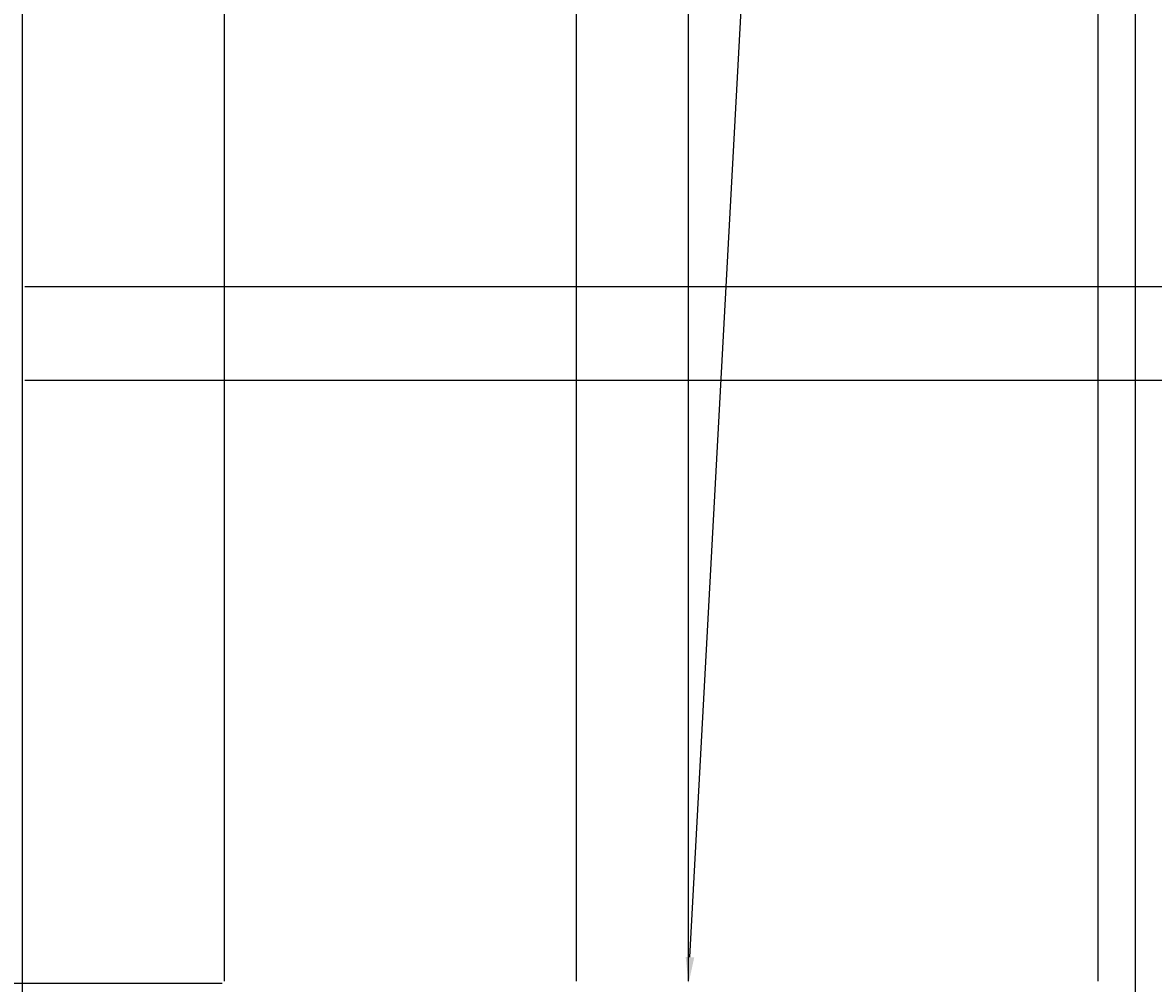
# Model space of a CAD drawing. Units: inches. Extents: x -12 to 334, y -10 to 186.
# Tile 23 of 77: x 58 to 88, y 109 to 135. Entities that reach past the tile are written whole.
import ezdxf
from ezdxf import colors
from ezdxf.entities.mleader import LeaderData, LeaderLine
from ezdxf.math import Vec2, Vec3

# ---------------------------------------------------------------- set-up
doc = ezdxf.new("R2010")
doc.units = ezdxf.units.IN
doc.header["$MEASUREMENT"] = 0
doc.layers.add('M-ANNO-TEXT', color=3, linetype='Continuous', lineweight=25)
doc.layers.add('M-DIMS', color=2, linetype='Continuous', lineweight=18)
doc.styles.get("Standard").update_dxf_attribs({"font": 'arial.ttf'})
doc.dimstyles.get("Standard").update_dxf_attribs({"dimtxt": 0.18, "dimasz": 0.18, "dimexe": 0.18, "dimexo": 0.0625, "dimgap": 0.09, "dimtad": 0, "dimtih": 1, "dimtoh": 1, "dimdec": 4, "dimzin": 0, "dimdsep": 46, "dimtxsty": 'Standard', "dimcen": 0.09, "dimadec": 0, "dimazin": 0, "dimtfac": 1, "dimtdec": 4, "dimtofl": 0, "dimtmove": 0, "dimatfit": 3, "dimfxl": 1, "dimtolj": 1, "dimtzin": 0, "dimarcsym": 0})

# ---------------------------------------------------------------- blocks, each defined once
blk = doc.blocks.new('*D3')
at = {"layer": 'Defpoints', "color": 0, "transparency": 16777216}
for p in [(58.1, 169.385), (32.1, 127.708), (58.1, 127.708)]:
    blk.add_point(p, dxfattribs=at)
at = {"layer": 'M-DIMS', "color": 0, "lineweight": -2, "transparency": 16777216}
for p, q in [((32.1, 127.77), (32.1, 169.565)), ((58.1, 127.77), (58.1, 169.565)), ((32.28, 169.385), (44.88, 169.385)), ((57.92, 169.385), (45.321, 169.385))]:
    blk.add_line(p, q, dxfattribs=at)
at = {"layer": 'M-DIMS', "color": 0, "transparency": 16777216}
for points in [[(32.28, 169.415), (32.28, 169.355), (32.1, 169.385)], [(57.92, 169.415), (57.92, 169.355), (58.1, 169.385)]]:
    blk.add_solid(points, dxfattribs=at)
at = {"layer": 'M-DIMS', "color": 0, "transparency": 16777216, "insert": (45.1, 169.385), "char_height": 0.18, "attachment_point": 5}
blk.add_mtext('\\A1;26', dxfattribs=at)
blk = doc.blocks.new('*D5')
at = {"layer": 'Defpoints', "color": 0, "transparency": 16777216}
for p in [(58.1, 127.708), (58.1, 125.208), (295.976, 125.208)]:
    blk.add_point(p, dxfattribs=at)
at = {"layer": 'M-DIMS', "color": 0, "lineweight": -2, "transparency": 16777216}
for p, q in [((58.163, 127.708), (296.156, 127.708)), ((295.976, 127.528), (295.976, 126.64)), ((295.976, 125.388), (295.976, 126.276)), ((58.163, 125.208), (296.156, 125.208))]:
    blk.add_line(p, q, dxfattribs=at)
at = {"layer": 'M-DIMS', "color": 0, "transparency": 16777216}
for points in [[(295.946, 127.528), (296.006, 127.528), (295.976, 127.708)], [(295.946, 125.388), (296.006, 125.388), (295.976, 125.208)]]:
    blk.add_solid(points, dxfattribs=at)
at = {"layer": 'M-DIMS', "color": 0, "transparency": 16777216, "insert": (295.976, 126.458), "char_height": 0.18, "attachment_point": 5}
blk.add_mtext('\\A1;2.5', dxfattribs=at)
blk = doc.blocks.new('*D10')
at = {"layer": 'Defpoints', "color": 0, "transparency": 16777216}
for p in [(63.5, 169.385), (58.1, 127.708), (63.5, 109.058)]:
    blk.add_point(p, dxfattribs=at)
at = {"layer": 'M-DIMS', "color": 0, "lineweight": -2, "transparency": 16777216}
for p, q in [((58.1, 127.77), (58.1, 169.565)), ((63.5, 109.121), (63.5, 169.565)), ((58.28, 169.385), (60.547, 169.385)), ((63.32, 169.385), (61.054, 169.385))]:
    blk.add_line(p, q, dxfattribs=at)
at = {"layer": 'M-DIMS', "color": 0, "transparency": 16777216}
for points in [[(58.28, 169.415), (58.28, 169.355), (58.1, 169.385)], [(63.32, 169.415), (63.32, 169.355), (63.5, 169.385)]]:
    blk.add_solid(points, dxfattribs=at)
at = {"layer": 'M-DIMS', "color": 0, "transparency": 16777216, "insert": (60.8, 169.385), "char_height": 0.18, "attachment_point": 5}
blk.add_mtext('\\A1;5.4', dxfattribs=at)
blk = doc.blocks.new('*D11')
at = {"layer": 'Defpoints', "color": 0, "transparency": 16777216}
for p in [(72.924, 169.385), (63.5, 109.058), (72.924, 109.058)]:
    blk.add_point(p, dxfattribs=at)
at = {"layer": 'M-DIMS', "color": 0, "lineweight": -2, "transparency": 16777216}
for p, q in [((63.5, 109.121), (63.5, 169.565)), ((72.924, 109.121), (72.924, 169.565)), ((63.68, 169.385), (67.819, 169.385)), ((72.744, 169.385), (68.606, 169.385))]:
    blk.add_line(p, q, dxfattribs=at)
at = {"layer": 'M-DIMS', "color": 0, "transparency": 16777216}
for points in [[(63.68, 169.415), (63.68, 169.355), (63.5, 169.385)], [(72.744, 169.415), (72.744, 169.355), (72.924, 169.385)]]:
    blk.add_solid(points, dxfattribs=at)
at = {"layer": 'M-DIMS', "color": 0, "transparency": 16777216, "insert": (68.212, 169.385), "char_height": 0.18, "attachment_point": 5}
blk.add_mtext('\\A1;9.424', dxfattribs=at)
blk = doc.blocks.new('*D12')
at = {"layer": 'Defpoints', "color": 0, "transparency": 16777216}
for p in [(75.924, 169.385), (72.924, 109.058), (75.924, 109.058)]:
    blk.add_point(p, dxfattribs=at)
at = {"layer": 'M-DIMS', "color": 0, "lineweight": -2, "transparency": 16777216}
for p, q in [((72.924, 109.121), (72.924, 169.565)), ((75.924, 109.121), (75.924, 169.565)), ((73.104, 169.385), (74.275, 169.385)), ((75.744, 169.385), (74.573, 169.385))]:
    blk.add_line(p, q, dxfattribs=at)
at = {"layer": 'M-DIMS', "color": 0, "transparency": 16777216}
for points in [[(73.104, 169.415), (73.104, 169.355), (72.924, 169.385)], [(75.744, 169.415), (75.744, 169.355), (75.924, 169.385)]]:
    blk.add_solid(points, dxfattribs=at)
at = {"layer": 'M-DIMS', "color": 0, "transparency": 16777216, "insert": (74.424, 169.385), "char_height": 0.18, "attachment_point": 5}
blk.add_mtext('\\A1;3', dxfattribs=at)
blk = doc.blocks.new('*D13')
at = {"layer": 'Defpoints', "color": 0, "transparency": 16777216}
for p in [(86.888, 169.385), (75.924, 109.058), (86.888, 109.058)]:
    blk.add_point(p, dxfattribs=at)
at = {"layer": 'M-DIMS', "color": 0, "lineweight": -2, "transparency": 16777216}
for p, q in [((75.924, 109.121), (75.924, 169.565)), ((86.888, 109.121), (86.888, 169.565)), ((76.104, 169.385), (80.951, 169.385)), ((86.708, 169.385), (81.861, 169.385))]:
    blk.add_line(p, q, dxfattribs=at)
at = {"layer": 'M-DIMS', "color": 0, "transparency": 16777216}
for points in [[(76.104, 169.415), (76.104, 169.355), (75.924, 169.385)], [(86.708, 169.415), (86.708, 169.355), (86.888, 169.385)]]:
    blk.add_solid(points, dxfattribs=at)
at = {"layer": 'M-DIMS', "color": 0, "transparency": 16777216, "insert": (81.406, 169.385), "char_height": 0.18, "attachment_point": 5}
blk.add_mtext('\\A1;10.964', dxfattribs=at)
blk = doc.blocks.new('*D14')
at = {"layer": 'Defpoints', "color": 0, "transparency": 16777216}
for p in [(63.5, 109.058), (-11.174, 49.45), (64.207, 49.45)]:
    blk.add_point(p, dxfattribs=at)
at = {"layer": 'M-DIMS', "color": 0, "lineweight": -2, "transparency": 16777216}
for p, q in [((63.438, 109.058), (-11.354, 109.058)), ((-11.174, 108.878), (-11.174, 79.436)), ((-11.174, 49.63), (-11.174, 79.072)), ((64.144, 49.45), (-11.354, 49.45))]:
    blk.add_line(p, q, dxfattribs=at)
at = {"layer": 'M-DIMS', "color": 0, "transparency": 16777216}
for points in [[(-11.204, 108.878), (-11.144, 108.878), (-11.174, 109.058)], [(-11.204, 49.63), (-11.144, 49.63), (-11.174, 49.45)]]:
    blk.add_solid(points, dxfattribs=at)
at = {"layer": 'M-DIMS', "color": 0, "transparency": 16777216, "insert": (-11.174, 79.254), "char_height": 0.18, "attachment_point": 5}
blk.add_mtext('\\A1;59.61', dxfattribs=at)
blk = doc.blocks.new('*D15')
at = {"layer": 'Defpoints', "color": 0, "transparency": 16777216}
for p in [(106.177, 169.385), (86.888, 109.058), (106.177, 102.896)]:
    blk.add_point(p, dxfattribs=at)
at = {"layer": 'M-DIMS', "color": 0, "lineweight": -2, "transparency": 16777216}
for p, q in [((86.888, 109.121), (86.888, 169.565)), ((106.177, 102.958), (106.177, 169.565)), ((87.068, 169.385), (96.147, 169.385)), ((105.997, 169.385), (96.918, 169.385))]:
    blk.add_line(p, q, dxfattribs=at)
at = {"layer": 'M-DIMS', "color": 0, "transparency": 16777216}
for points in [[(87.068, 169.415), (87.068, 169.355), (86.888, 169.385)], [(105.997, 169.415), (105.997, 169.355), (106.177, 169.385)]]:
    blk.add_solid(points, dxfattribs=at)
at = {"layer": 'M-DIMS', "color": 0, "transparency": 16777216, "insert": (96.532, 169.385), "char_height": 0.18, "attachment_point": 5}
blk.add_mtext('\\A1;19.29', dxfattribs=at)
blk = doc.blocks.new('*D26')
at = {"layer": 'Defpoints', "color": 0, "transparency": 16777216}
for p in [(87.888, 169.385), (87.888, 56.321), (58.1, 33.675)]:
    blk.add_point(p, dxfattribs=at)
at = {"layer": 'M-DIMS', "color": 0, "lineweight": -2, "transparency": 16777216}
for p, q in [((58.1, 33.738), (58.1, 169.565)), ((87.888, 56.383), (87.888, 169.565)), ((58.28, 169.385), (72.599, 169.385)), ((87.708, 169.385), (73.389, 169.385))]:
    blk.add_line(p, q, dxfattribs=at)
at = {"layer": 'M-DIMS', "color": 0, "transparency": 16777216}
for points in [[(58.28, 169.415), (58.28, 169.355), (58.1, 169.385)], [(87.708, 169.415), (87.708, 169.355), (87.888, 169.385)]]:
    blk.add_solid(points, dxfattribs=at)
at = {"layer": 'M-DIMS', "color": 0, "transparency": 16777216, "insert": (72.994, 169.385), "char_height": 0.18, "attachment_point": 5}
blk.add_mtext('\\A1;29.79', dxfattribs=at)

msp = doc.modelspace()

# ---------------------------------------------------------------- dimensions: what is measured, and where the dimension line sits
at = {"layer": 'M-DIMS'}
for base, p1, p2, override, picture, middle in [((58.1002, 169.3845), (32.1002, 127.7078), (58.1002, 127.7078), {"dimdec": 0, "dimlfac": 1, "dimrnd": 0, "dimzin": 0, "dimdsep": 46, "dimlunit": 2}, '*D3', (45.1002, 169.3845)), ((63.5, 169.3845), (58.1002, 127.7078), (63.5, 109.0583), {"dimdec": 1, "dimlfac": 1, "dimrnd": 0, "dimzin": 0, "dimdsep": 46, "dimlunit": 2}, '*D10', (60.8001, 169.3845)), ((87.8879, 169.3845), (58.1002, 33.6752), (87.8879, 56.3205), {"dimdec": 2, "dimlfac": 1, "dimrnd": 0, "dimzin": 0, "dimdsep": 46, "dimlunit": 2}, '*D26', (72.9941, 169.3845)), ((72.9244, 169.3845), (63.5, 109.0583), (72.9244, 109.0583), {"dimdec": 3, "dimlfac": 1, "dimrnd": 0, "dimzin": 0, "dimdsep": 46, "dimlunit": 2}, '*D11', (68.2122, 169.3845)), ((75.9244, 169.3845), (72.9244, 109.0583), (75.9244, 109.0583), {"dimdec": 0, "dimlfac": 1, "dimrnd": 0, "dimzin": 0, "dimdsep": 46, "dimlunit": 2}, '*D12', (74.4244, 169.3845)), ((86.887907, 169.384532), (75.924407, 109.05834), (86.887907, 109.05834), {"dimdec": 3, "dimlfac": 1, "dimrnd": 0, "dimzin": 0, "dimdsep": 46, "dimlunit": 2}, '*D13', (81.406157, 169.384532)), ((106.1771, 169.3845), (86.8879, 109.0583), (106.1771, 102.8958), {"dimdec": 2, "dimlfac": 1, "dimrnd": 0, "dimzin": 0, "dimdsep": 46, "dimlunit": 2}, '*D15', (96.5325, 169.3845))]:
    dim = msp.add_linear_dim(base=base, p1=p1, p2=p2, dimstyle='Standard', override=override, dxfattribs=at)
    dim.commit()
    dim.dimension.update_dxf_attribs({"geometry": picture, "text_midpoint": middle})
for base, p1, p2, override, picture, middle in [((295.9756, 125.2078), (58.1002, 127.7078), (58.1002, 125.2078), {"dimdec": 1, "dimlfac": 1, "dimrnd": 0, "dimzin": 0, "dimdsep": 46, "dimlunit": 2}, '*D5', (295.9756, 126.4578)), ((-11.1736, 49.4497), (63.5, 109.0583), (64.2068, 49.4497), {"dimdec": 2, "dimlfac": 1, "dimrnd": 0, "dimzin": 0, "dimdsep": 46, "dimlunit": 2}, '*D14', (-11.1735, 79.254))]:
    dim = msp.add_linear_dim(base=base, p1=p1, p2=p2, angle=90, dimstyle='Standard', override=override, dxfattribs=at)
    dim.commit()
    dim.dimension.update_dxf_attribs({"geometry": picture, "text_midpoint": middle})

# ---------------------------------------------------------------- leaders
at = {"layer": 'M-ANNO-TEXT'}
ml = msp.add_multileader_mtext('Standard', dxfattribs=at)
ml.set_content('Tube plate', color=256)
ml.set_leader_properties()
ml.build(insert=Vec2(0, 0))
ml.multileader.update_dxf_attribs({"dogleg_length": 0.36, "arrow_head_size": 0.7})
ctx = ml.context
ctx.base_point, ctx.arrow_head_size, ctx.landing_gap_size, ctx.plane_origin = Vec3(95.9742, 157.4218), 0.7, 0.09, Vec3(31.4743, 171.7024)
notes = []
notes.append((ctx, [(0, (1, 1, 0), (78.5354, 157.4218), (1, 0), 17.4388, [(0, [(75.9244, 109.0583)], 0, [])])]))
ctx.mtext.insert, ctx.mtext.flow_direction = Vec3(96.0642, 159.9771), 5
for ctx, leaders in notes:
    for number, flags, end, landing, length, lines in leaders:
        leader = LeaderData()
        leader.index, (leader.has_last_leader_line, leader.has_dogleg_vector, leader.attachment_direction) = number, flags
        leader.last_leader_point, leader.dogleg_vector, leader.dogleg_length = Vec3(end), Vec3(landing), length
        for number, points, colour, breaks in lines:
            line = LeaderLine()
            line.index, line.vertices, line.color, line.breaks = number, Vec3.list(points), colors.encode_raw_color(colour), breaks
            leader.lines.append(line)
        ctx.leaders.append(leader)

doc.saveas('drawing.dxf')
